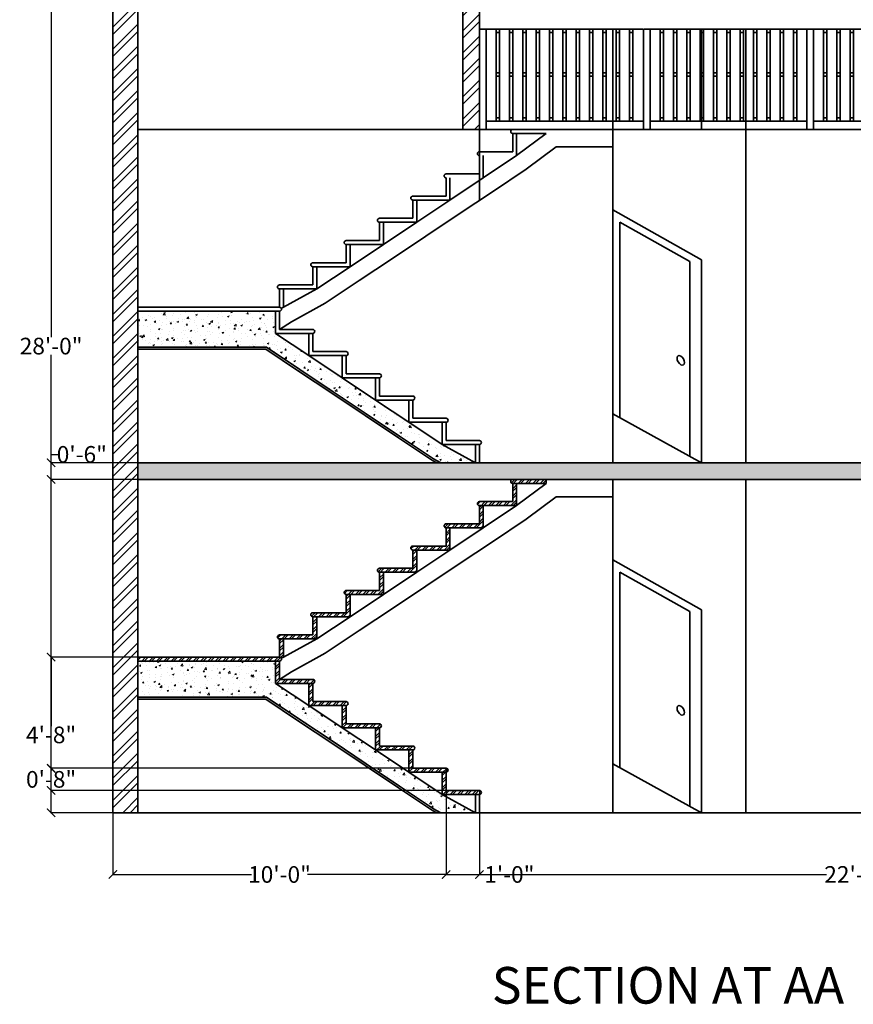
# Model space of a CAD drawing. Units: inches. Extents: x 2278 to 7495, y -71 to 1198.
# Tile 39 of 44: x 6954 to 7254, y 85 to 439. Entities that reach past the tile are written whole.
import ezdxf

# ---------------------------------------------------------------- set-up
doc = ezdxf.new("R2010")
doc.units = ezdxf.units.IN
doc.header["$MEASUREMENT"] = 0
for name, color, linetype, lineweight in [('A-ANNO-DIMS', 2, 'Continuous', 18), ('A-ANNO-TEXT', 7, 'Continuous', 25), ('A-SECT', 7, 'Continuous', 35), ('A-SECT-PATT', 8, 'Continuous', 13)]:
    doc.layers.add(name, color=color, linetype=linetype, lineweight=lineweight)
doc.styles.add('ATTR', font='romans.shx', dxfattribs={"width": 0.8, "height": 0.7})
doc.styles.get("Standard").update_dxf_attribs({"font": 'arial.ttf'})
doc.dimstyles.get("Standard").update_dxf_attribs({"dimtxt": 6, "dimasz": 3, "dimexe": 0.18, "dimexo": 0.0625, "dimgap": 0.09, "dimtad": 0, "dimtih": 1, "dimtoh": 1, "dimdec": 0, "dimzin": 0, "dimdsep": 46, "dimlunit": 3, "dimtxsty": 'Standard', "dimblk": 'ARCHTICK', "dimcen": 0.09, "dimadec": 0, "dimazin": 0, "dimtfac": 1, "dimtdec": 0, "dimtofl": 0, "dimtmove": 0, "dimatfit": 3, "dimfxl": 1, "dimtolj": 1, "dimtzin": 0, "dimarcsym": 0})
pattern_1 = [(45, (0, 155.5801), (-1.3258252, 1.3258252), []), (45, (0.8839, 155.5801), (-1.3258252, 1.3258252), [])]
pattern_2 = [(50, (0, 155.58), (5.7380815, -0.502017), [0.6, -6.6]), (355, (0, 155.58), (-1.1100107, 6.017537), [0.48, -5.28]), (100.45144, (0.478, 155.538), (4.6280708, 5.51552), [0.5099215, -5.609137]), (46.1842, (0, 157.18), (8.5379306, -1.324154), [0.9, -9.9]), (96.63564, (0.7115, 157.07), (7.477296, 7.792949), [0.764883, -8.41371]), (351.18416, (0, 157.18), (7.477296, 7.792949), [0.72, -7.92]), (21, (0.8, 156.78), (4.7752564, -3.220951), [0.6, -6.6]), (326, (0.8, 156.78), (1.9465227, 5.8012004), [0.48, -5.28]), (71.451445, (1.198, 156.5117), (6.721779, 2.5802492), [0.5099215, -5.609137]), (37.5, (0, 155.5801), (0.09727884, 2.66315083), [0, -5.216, 0, -5.36, 0, -5.3]), (7.5, (0, 155.58), (2.1045563, 3.1552937), [0, -3.056, 0, -5.096, 0, -2.02]), (327.5, (-1.784, 155.5801), (4.2705795, -0.180439), [0, -2, 0, -6.24, 0, -8.28]), (317.5, (-2.584, 155.58), (4.6654894, 0.8008399), [0, -2.6, 0, -4.144, 0, -5.88])]

# ---------------------------------------------------------------- blocks, each defined once
blk = doc.blocks.new('Fence 2 EV')
for p, q in [((0, 60), (0, 0)), ((0.001, 60.008), (98.001, 60.008)), ((4, 0.002), (4, 60)), ((10, 60), (10, 5.002)), ((12, 60), (12, 5.002)), ((18, 5.002), (18, 60)), ((20, 60), (20, 5.002)), ((25.999, 5.002), (25.999, 60)), ((27.999, 60), (27.999, 5.002)), ((33.999, 5.002), (33.999, 60)), ((35.999, 60), (35.999, 5.002)), ((41.999, 5.002), (41.999, 60)), ((43.999, 60), (43.999, 5.002)), ((49.999, 5.002), (49.999, 60)), ((51.998, 60), (51.998, 5.002)), ((57.998, 5.002), (57.998, 60)), ((59.998, 60), (59.998, 5.002)), ((65.998, 5.002), (65.998, 60)), ((67.998, 60), (67.998, 5.002)), ((73.998, 5.002), (73.998, 60)), ((75.997, 60), (75.997, 5.002)), ((81.997, 5.002), (81.997, 60)), ((83.997, 60), (83.997, 5.002)), ((89.997, 5.002), (89.997, 60)), ((91.997, 60), (91.997, 5.002)), ((10, 58), (12, 58)), ((18, 58), (20, 58)), ((25.999, 58), (27.999, 58)), ((33.999, 58), (35.999, 58)), ((41.999, 58), (43.999, 58)), ((49.999, 58), (51.998, 58)), ((57.998, 58), (59.998, 58)), ((65.998, 58), (67.998, 58)), ((73.998, 58), (75.997, 58)), ((81.997, 58), (83.997, 58)), ((89.997, 58), (91.997, 58)), ((10, 34.001), (12, 34.001)), ((10, 32.001), (12, 32.001)), ((18, 34.001), (20, 34.001)), ((18, 32.001), (20, 32.001)), ((25.999, 34.001), (27.999, 34.001)), ((25.999, 32.001), (27.999, 32.001)), ((33.999, 34.001), (35.999, 34.001)), ((33.999, 32.001), (35.999, 32.001)), ((41.999, 34.001), (43.999, 34.001)), ((41.999, 32.001), (43.999, 32.001)), ((49.999, 34.001), (51.998, 34.001)), ((49.999, 32.001), (51.998, 32.001)), ((57.998, 34.001), (59.998, 34.001)), ((57.998, 32.001), (59.998, 32.001)), ((65.998, 34.001), (67.998, 34.001)), ((65.998, 32.001), (67.998, 32.001)), ((73.998, 34.001), (75.997, 34.001)), ((73.998, 32.001), (75.997, 32.001)), ((81.997, 34.001), (83.997, 34.001)), ((81.997, 32.001), (83.997, 32.001)), ((89.997, 34.001), (91.997, 34.001)), ((89.997, 32.001), (91.997, 32.001)), ((10, 7.002), (12, 7.002)), ((18, 7.002), (20, 7.002)), ((25.999, 7.002), (27.999, 7.002)), ((33.999, 7.002), (35.999, 7.002)), ((41.999, 7.002), (43.999, 7.002)), ((49.999, 7.002), (51.998, 7.002)), ((57.998, 7.002), (59.998, 7.002)), ((65.998, 7.002), (67.998, 7.002)), ((73.998, 7.002), (75.997, 7.002)), ((81.997, 7.002), (83.997, 7.002)), ((89.997, 7.002), (91.997, 7.002)), ((0, 0.002), (4, 0.002)), ((97.997, 5.002), (4, 5.002))]:
    blk.add_line(p, q)
at = {"style": 'ATTR', "width": 0.8, "flags": 9}
blk.add_attdef('ESTCODE', (0, 0), '', height=0.0196, dxfattribs=at)
blk = doc.blocks.new('_ArchTick')
at = {"color": 0, "linetype": 'ByBlock', "const_width": 0.15}
blk.add_lwpolyline([(-0.5, -0.5), (0.5, 0.5)], dxfattribs=at)
blk = doc.blocks.new('*D113')
at = {"layer": 'A-ANNO-DIMS', "color": 0, "lineweight": -2, "transparency": 16777216}
for p, q in [((7119.18, 489.83), (7412.55, 489.83)), ((7412.37, 489.83), (7412.37, 447.99)), ((7412.37, 399.83), (7412.37, 441.68)), ((7119.18, 399.83), (7412.55, 399.83))]:
    blk.add_line(p, q, dxfattribs=at)
at = {"layer": 'Defpoints', "color": 0, "transparency": 16777216}
for p in [(7119.12, 489.83), (7412.37, 489.83), (7119.12, 399.83)]:
    blk.add_point(p, dxfattribs=at)
at = {"layer": 'A-ANNO-DIMS', "color": 0, "lineweight": -2, "transparency": 16777216, "xscale": 3, "yscale": 3, "zscale": 3}
for p, rotation in [((7412.37, 489.83), 90), ((7412.37, 399.83), 270)]:
    blk.add_blockref('_ArchTick', p, dxfattribs=dict(at, rotation=rotation))
at = {"layer": 'A-ANNO-DIMS', "color": 0, "transparency": 16777216, "insert": (7412.37, 444.83), "char_height": 6, "attachment_point": 5}
blk.add_mtext('\\A1;7\'-6"', dxfattribs=at)
blk = doc.blocks.new('*D114')
at = {"layer": 'A-ANNO-DIMS', "color": 0, "lineweight": -2, "transparency": 16777216}
for p, q in [((6987.05, 489.83), (6964.69, 489.83)), ((6964.87, 489.83), (6964.87, 324.99)), ((6964.87, 153.83), (6964.87, 318.68)), ((6987.05, 153.83), (6964.69, 153.83))]:
    blk.add_line(p, q, dxfattribs=at)
at = {"layer": 'Defpoints', "color": 0, "transparency": 16777216}
for p in [(6964.87, 489.83), (6987.12, 489.83), (6987.12, 153.83)]:
    blk.add_point(p, dxfattribs=at)
at = {"layer": 'A-ANNO-DIMS', "color": 0, "lineweight": -2, "transparency": 16777216, "xscale": 3, "yscale": 3, "zscale": 3}
for p, rotation in [((6964.87, 489.83), 90), ((6964.87, 153.83), 270)]:
    blk.add_blockref('_ArchTick', p, dxfattribs=dict(at, rotation=rotation))
at = {"layer": 'A-ANNO-DIMS', "color": 0, "transparency": 16777216, "insert": (6964.87, 321.83), "char_height": 6, "attachment_point": 5}
blk.add_mtext('\\A1;28\'-0"', dxfattribs=at)
blk = doc.blocks.new('*D115')
at = {"layer": 'A-ANNO-DIMS', "color": 0, "lineweight": -2, "transparency": 16777216}
for p, q in [((6996.05, 209.83), (6964.69, 209.83)), ((6964.87, 209.83), (6964.87, 184.99)), ((6964.87, 153.83), (6964.87, 178.68)), ((6996.05, 153.83), (6964.69, 153.83))]:
    blk.add_line(p, q, dxfattribs=at)
at = {"layer": 'Defpoints', "color": 0, "transparency": 16777216}
for p in [(6964.87, 209.83), (6996.12, 209.83), (6996.12, 153.83)]:
    blk.add_point(p, dxfattribs=at)
at = {"layer": 'A-ANNO-DIMS', "color": 0, "lineweight": -2, "transparency": 16777216, "xscale": 3, "yscale": 3, "zscale": 3}
for p, rotation in [((6964.87, 209.83), 90), ((6964.87, 153.83), 270)]:
    blk.add_blockref('_ArchTick', p, dxfattribs=dict(at, rotation=rotation))
at = {"layer": 'A-ANNO-DIMS', "color": 0, "transparency": 16777216, "insert": (6964.87, 181.83), "char_height": 6, "attachment_point": 5}
blk.add_mtext('\\A1;4\'-8"', dxfattribs=at)
blk = doc.blocks.new('*D116')
at = {"layer": 'A-ANNO-DIMS', "color": 0, "lineweight": -2, "transparency": 16777216}
for p, q in [((6964.87, 279.83), (6964.87, 282.83)), ((6964.87, 282.83), (6967.87, 282.83)), ((6996.05, 279.83), (6964.69, 279.83)), ((6964.87, 273.83), (6964.87, 279.83)), ((6996.05, 273.83), (6964.69, 273.83))]:
    blk.add_line(p, q, dxfattribs=at)
at = {"layer": 'Defpoints', "color": 0, "transparency": 16777216}
for p in [(6964.87, 279.83), (6996.12, 279.83), (6996.12, 273.83)]:
    blk.add_point(p, dxfattribs=at)
at = {"layer": 'A-ANNO-DIMS', "color": 0, "lineweight": -2, "transparency": 16777216, "xscale": 3, "yscale": 3, "zscale": 3}
for p, rotation in [((6964.87, 279.83), 90), ((6964.87, 273.83), 270)]:
    blk.add_blockref('_ArchTick', p, dxfattribs=dict(at, rotation=rotation))
at = {"layer": 'A-ANNO-DIMS', "color": 0, "transparency": 16777216, "insert": (6975.93, 282.83), "char_height": 6, "attachment_point": 5}
blk.add_mtext('\\A1;0\'-6"', dxfattribs=at)
blk = doc.blocks.new('*D117')
at = {"layer": 'A-ANNO-DIMS', "color": 0, "lineweight": -2, "transparency": 16777216}
for p, q in [((7107.05, 169.83), (6964.69, 169.83)), ((6964.87, 169.83), (6964.87, 168.99)), ((7119.05, 161.83), (6964.69, 161.83)), ((6964.87, 161.83), (6964.87, 162.68))]:
    blk.add_line(p, q, dxfattribs=at)
at = {"layer": 'Defpoints', "color": 0, "transparency": 16777216}
for p in [(6964.87, 169.83), (7107.12, 169.83), (7119.12, 161.83)]:
    blk.add_point(p, dxfattribs=at)
at = {"layer": 'A-ANNO-DIMS', "color": 0, "lineweight": -2, "transparency": 16777216, "xscale": 3, "yscale": 3, "zscale": 3}
for p, rotation in [((6964.87, 169.83), 90), ((6964.87, 161.83), 270)]:
    blk.add_blockref('_ArchTick', p, dxfattribs=dict(at, rotation=rotation))
at = {"layer": 'A-ANNO-DIMS', "color": 0, "transparency": 16777216, "insert": (6964.87, 165.83), "char_height": 6, "attachment_point": 5}
blk.add_mtext('\\A1;0\'-8"', dxfattribs=at)
blk = doc.blocks.new('*D118')
at = {"layer": 'A-ANNO-DIMS', "color": 0, "lineweight": -2, "transparency": 16777216}
for p, q in [((7107.12, 169.77), (7107.12, 131.4)), ((6987.12, 153.77), (6987.12, 131.4)), ((6987.12, 131.58), (7037, 131.58)), ((7107.12, 131.58), (7057.23, 131.58))]:
    blk.add_line(p, q, dxfattribs=at)
at = {"layer": 'Defpoints', "color": 0, "transparency": 16777216}
for p in [(7107.12, 169.83), (6987.12, 153.83), (7107.12, 131.58)]:
    blk.add_point(p, dxfattribs=at)
at = {"layer": 'A-ANNO-DIMS', "color": 0, "lineweight": -2, "transparency": 16777216, "xscale": 3, "yscale": 3, "zscale": 3, "rotation": 180}
blk.add_blockref('_ArchTick', (6987.12, 131.58), dxfattribs=at)
at = {"layer": 'A-ANNO-DIMS', "color": 0, "lineweight": -2, "transparency": 16777216, "xscale": 3, "yscale": 3, "zscale": 3}
blk.add_blockref('_ArchTick', (7107.12, 131.58), dxfattribs=at)
at = {"layer": 'A-ANNO-DIMS', "color": 0, "transparency": 16777216, "insert": (7047.12, 131.58), "char_height": 6, "attachment_point": 5}
blk.add_mtext('\\A1;10\'-0"', dxfattribs=at)
blk = doc.blocks.new('*D119')
at = {"layer": 'A-ANNO-DIMS', "color": 0, "lineweight": -2, "transparency": 16777216}
for p, q in [((7107.12, 169.77), (7107.12, 131.4)), ((7119.12, 161.77), (7119.12, 131.4)), ((7107.12, 131.58), (7119.12, 131.58)), ((7119.12, 131.58), (7122.12, 131.58))]:
    blk.add_line(p, q, dxfattribs=at)
at = {"layer": 'Defpoints', "color": 0, "transparency": 16777216}
for p in [(7107.12, 169.83), (7119.12, 161.83), (7119.12, 131.58)]:
    blk.add_point(p, dxfattribs=at)
at = {"layer": 'A-ANNO-DIMS', "color": 0, "lineweight": -2, "transparency": 16777216, "xscale": 3, "yscale": 3, "zscale": 3, "rotation": 180}
blk.add_blockref('_ArchTick', (7107.12, 131.58), dxfattribs=at)
at = {"layer": 'A-ANNO-DIMS', "color": 0, "lineweight": -2, "transparency": 16777216, "xscale": 3, "yscale": 3, "zscale": 3}
blk.add_blockref('_ArchTick', (7119.12, 131.58), dxfattribs=at)
at = {"layer": 'A-ANNO-DIMS', "color": 0, "transparency": 16777216, "insert": (7129.9, 131.58), "char_height": 6, "attachment_point": 5}
blk.add_mtext('\\A1;1\'-0"', dxfattribs=at)
blk = doc.blocks.new('*D120')
at = {"layer": 'A-ANNO-DIMS', "color": 0, "lineweight": -2, "transparency": 16777216}
for p, q in [((7119.12, 161.77), (7119.12, 131.4)), ((7390.12, 153.77), (7390.12, 131.4)), ((7119.12, 131.58), (7244.17, 131.58)), ((7390.12, 131.58), (7265.06, 131.58))]:
    blk.add_line(p, q, dxfattribs=at)
at = {"layer": 'Defpoints', "color": 0, "transparency": 16777216}
for p in [(7119.12, 161.83), (7390.12, 153.83), (7390.12, 131.58)]:
    blk.add_point(p, dxfattribs=at)
at = {"layer": 'A-ANNO-DIMS', "color": 0, "lineweight": -2, "transparency": 16777216, "xscale": 3, "yscale": 3, "zscale": 3, "rotation": 180}
blk.add_blockref('_ArchTick', (7119.12, 131.58), dxfattribs=at)
at = {"layer": 'A-ANNO-DIMS', "color": 0, "lineweight": -2, "transparency": 16777216, "xscale": 3, "yscale": 3, "zscale": 3}
blk.add_blockref('_ArchTick', (7390.12, 131.58), dxfattribs=at)
at = {"layer": 'A-ANNO-DIMS', "color": 0, "transparency": 16777216, "insert": (7254.62, 131.58), "char_height": 6, "attachment_point": 5}
blk.add_mtext('\\A1;22\'-7"', dxfattribs=at)
blk = doc.blocks.new('*D122')
at = {"layer": 'A-ANNO-DIMS', "color": 0, "lineweight": -2, "transparency": 16777216}
for p, q in [((7119.12, 489.9), (7119.12, 512.26)), ((7119.12, 512.08), (7244.17, 512.08)), ((7390.11, 512.08), (7265.06, 512.08)), ((7390.11, 435.95), (7390.11, 512.26))]:
    blk.add_line(p, q, dxfattribs=at)
at = {"layer": 'Defpoints', "color": 0, "transparency": 16777216}
for p in [(7390.11, 512.08), (7119.12, 489.83), (7390.11, 435.89)]:
    blk.add_point(p, dxfattribs=at)
at = {"layer": 'A-ANNO-DIMS', "color": 0, "lineweight": -2, "transparency": 16777216, "xscale": 3, "yscale": 3, "zscale": 3, "rotation": 180}
blk.add_blockref('_ArchTick', (7119.12, 512.08), dxfattribs=at)
at = {"layer": 'A-ANNO-DIMS', "color": 0, "lineweight": -2, "transparency": 16777216, "xscale": 3, "yscale": 3, "zscale": 3}
blk.add_blockref('_ArchTick', (7390.11, 512.08), dxfattribs=at)
at = {"layer": 'A-ANNO-DIMS', "color": 0, "transparency": 16777216, "insert": (7254.61, 512.08), "char_height": 6, "attachment_point": 5}
blk.add_mtext('\\A1;22\'-7"', dxfattribs=at)

msp = doc.modelspace()

# ---------------------------------------------------------------- hatches: boundary and pattern name
at = {"layer": 'A-SECT-PATT', "transparency": 33554687}
h = msp.add_hatch(dxfattribs=at)
h.set_pattern_fill('ANSI32', color=256, scale=15)
h.set_pattern_definition([(45, (0, 155.58), (-3.9774756, 3.9774756), []), (45, (2.6517, 155.58), (-3.9774756, 3.9774756), [])])
h.paths.add_polyline_path([(6996.12, 489.83), (6987.12, 489.83), (6987.12, 153.83), (6996.12, 153.83)])
h.paths.add_polyline_path([(7390.12, 399.83), (7381.12, 399.83), (7381.12, 153.83), (7390.12, 153.83)])
h.paths.add_polyline_path([(7119.12, 483.83), (7119.12, 489.83), (7113.12, 489.83), (7113.12, 399.83), (7119.12, 399.83)])
h = msp.add_hatch(dxfattribs=at)
h.set_pattern_fill('AR-CONC', color=256, scale=0.8)
h.set_pattern_definition(pattern_2)
h.paths.add_polyline_path([(7045.72, 334.4), (6996.12, 334.4), (6996.12, 321.4), (7042.39, 321.4), (7054.39, 313.4), (7066.39, 305.4), (7078.39, 297.4), (7090.39, 289.4), (7102.61, 281.26), (7105.21, 279.83), (7117.72, 279.83), (7105.72, 286.4), (7093.72, 294.4), (7081.72, 302.4), (7069.72, 310.4), (7057.72, 318.4), (7045.72, 326.4)])
h = msp.add_hatch(dxfattribs=at)
h.set_pattern_fill('AR-CONC', color=256, scale=0.8)
h.set_pattern_definition([(50, (0, 0), (5.7380815, -0.502017), [0.6, -6.6]), (355, (0, 0), (-1.1100107, 6.017537), [0.48, -5.28]), (100.451444, (0.478, -0.042), (4.6280708, 5.51552), [0.5099215, -5.609137]), (46.1842, (0, 1.6), (8.5379306, -1.324154), [0.9, -9.9]), (96.63564, (0.7115, 1.49), (7.477296, 7.792949), [0.764883, -8.41371]), (351.18416, (0, 1.6), (7.477296, 7.792949), [0.72, -7.92]), (21, (0.8, 1.2), (4.7752564, -3.220951), [0.6, -6.6]), (326, (0.8, 1.2), (1.9465227, 5.8012004), [0.48, -5.28]), (71.451445, (1.198, 0.9316), (6.721779, 2.5802492), [0.5099215, -5.609137]), (37.5, (0, 0), (0.09727884, 2.66315083), [0, -5.216, 0, -5.36, 0, -5.3]), (7.5, (0, 0), (2.1045563, 3.1552937), [0, -3.056, 0, -5.096, 0, -2.02]), (327.5, (-1.784, 0), (4.2705795, -0.180439), [0, -2, 0, -6.24, 0, -8.28]), (317.5, (-2.584, 0), (4.6654894, 0.8008399), [0, -2.6, 0, -4.144, 0, -5.88])])
h.paths.add_polyline_path([(7381.12, 279.83), (6996.12, 279.83), (6996.12, 273.83), (7131.12, 273.83), (7143.12, 273.83), (7167.12, 273.83), (7381.12, 273.83)])
h = msp.add_hatch(dxfattribs=at)
h.set_pattern_fill('ANSI32', color=256, scale=5)
h.set_pattern_definition(pattern_1)
h.paths.add_polyline_path([(7143.12, 273.83), (7131.12, 273.83, 1), (7131.12, 272.4), (7143.12, 272.4)])
h = msp.add_hatch(dxfattribs=at)
h.set_pattern_fill('ANSI32', color=256, scale=5)
h.set_pattern_definition(pattern_1)
h.paths.add_polyline_path([(7107.12, 169.83), (7095.12, 169.83), (7095.12, 176.4), (7093.72, 176.4), (7093.72, 168.4), (7107.12, 168.4, 1)])
h.paths.add_polyline_path([(7107.12, 168.4), (7105.72, 168.4), (7105.72, 160.4), (7119.12, 160.4, 1), (7119.12, 161.83), (7107.12, 161.83)])
h.paths.add_polyline_path([(7095.12, 177.83), (7083.12, 177.83), (7083.12, 184.4), (7081.72, 184.4), (7081.72, 176.4), (7095.12, 176.4, 1)])
h.paths.add_polyline_path([(7083.12, 185.83), (7071.12, 185.83), (7071.12, 192.4), (7069.72, 192.4), (7069.72, 184.4), (7083.12, 184.4, 1)])
h.paths.add_polyline_path([(7071.12, 193.83), (7059.12, 193.83), (7059.12, 200.4), (7057.72, 200.4), (7057.72, 192.4), (7071.12, 192.4, 1)])
h.paths.add_polyline_path([(7059.12, 201.83), (7047.12, 201.83), (7047.12, 208.4), (7045.72, 208.4), (7045.72, 200.4), (7059.12, 200.4, 1)])
h.paths.add_polyline_path([(7047.12, 209.83), (7035.12, 209.83), (6996.12, 209.83), (6996.12, 208.4), (7047.12, 208.4, 1)])
h.paths.add_polyline_path([(7048.52, 216.4), (7047.12, 216.4), (7047.12, 209.83, -0.289905), (7047.76, 209.42), (7048.52, 209.83)])
h.paths.add_polyline_path([(7060.52, 224.4), (7059.12, 224.4), (7059.12, 217.83), (7047.12, 217.83, 1), (7047.12, 216.4), (7048.52, 216.4), (7060.52, 216.4)])
h.paths.add_polyline_path([(7072.52, 232.4), (7071.12, 232.4), (7071.12, 225.83), (7059.12, 225.83, 1), (7059.12, 224.4), (7060.52, 224.4), (7072.52, 224.4)])
h.paths.add_polyline_path([(7084.52, 240.4), (7083.12, 240.4), (7083.12, 233.83), (7071.12, 233.83, 1), (7071.12, 232.4), (7072.52, 232.4), (7084.52, 232.4)])
h.paths.add_polyline_path([(7096.52, 248.4), (7095.12, 248.4), (7095.12, 241.83), (7083.12, 241.83, 1), (7083.12, 240.4), (7084.52, 240.4), (7096.52, 240.4)])
h.paths.add_polyline_path([(7108.52, 256.4), (7107.12, 256.4), (7107.12, 249.83), (7095.12, 249.83, 1), (7095.12, 248.4), (7096.52, 248.4), (7108.52, 248.4)])
h.paths.add_polyline_path([(7120.52, 264.4), (7119.12, 264.4), (7119.12, 257.83), (7107.12, 257.83, 1), (7107.12, 256.4), (7120.52, 256.4)])
h.paths.add_polyline_path([(7132.52, 272.4), (7131.12, 272.4), (7131.12, 265.83), (7119.12, 265.83, 1), (7119.12, 264.4), (7120.52, 264.4), (7132.52, 264.4)])
h = msp.add_hatch(dxfattribs=at)
h.set_pattern_fill('AR-CONC', color=256, scale=0.8)
h.set_pattern_definition(pattern_2)
h.paths.add_polyline_path([(7045.72, 208.4), (6996.12, 208.4), (6996.12, 195.4), (7042.39, 195.4), (7054.39, 187.4), (7066.39, 179.4), (7078.39, 171.4), (7090.39, 163.4), (7102.61, 155.26), (7105.21, 153.83), (7117.72, 153.83), (7105.72, 160.4), (7093.72, 168.4), (7081.72, 176.4), (7069.72, 184.4), (7057.72, 192.4), (7045.72, 200.4)])

# ---------------------------------------------------------------- linework, layer by layer
at = {"layer": 'A-SECT'}
for p, q in [((6987.12, 153.83), (6987.12, 489.83)), ((6996.12, 153.83), (6996.12, 489.83)), ((7113.12, 399.83), (7113.12, 489.83)), ((7119.12, 489.83), (7119.12, 374.25)), ((7119.12, 399.83), (7119.12, 483.83)), ((7167.12, 435.89), (7167.12, 279.83)), ((7199.04, 399.83), (7199.04, 435.89)), ((7215.12, 435.89), (7215.12, 279.83)), ((6996.12, 399.83), (7390.12, 399.83)), ((7131.12, 399.83), (7143.12, 399.83)), ((7131.12, 398.4), (7131.12, 391.83)), ((7143.12, 398.4), (7131.12, 398.4)), ((7132.52, 398.4), (7132.52, 390.4)), ((7167.12, 393.61), (7167.12, 399.83)), ((7146.73, 393.61), (7167.12, 393.61)), ((7119.12, 391.83), (7131.12, 391.83)), ((7119.12, 390.4), (7119.12, 383.83)), ((7120.52, 390.4), (7120.52, 382.4)), ((7107.12, 383.83), (7119.12, 383.83)), ((7107.12, 382.4), (7107.12, 375.83)), ((7108.52, 382.4), (7108.52, 374.4)), ((7095.12, 375.83), (7107.12, 375.83)), ((7095.12, 374.4), (7095.12, 367.83)), ((7108.52, 374.4), (7095.12, 374.4)), ((7096.52, 374.4), (7096.52, 366.4)), ((7167.12, 297.43), (7167.12, 370.92)), ((7167.12, 370.92), (7199.04, 352.92)), ((7083.12, 367.83), (7095.12, 367.83)), ((7083.12, 366.4), (7083.12, 359.83)), ((7096.52, 366.4), (7083.12, 366.4)), ((7084.52, 366.4), (7084.52, 358.4)), ((7169.71, 366.46), (7194.85, 352.28)), ((7169.71, 295.93), (7169.71, 366.46)), ((7071.12, 359.83), (7083.12, 359.83)), ((7071.12, 358.4), (7071.12, 351.83)), ((7084.52, 358.4), (7071.12, 358.4)), ((7072.52, 358.4), (7072.52, 350.4)), ((7059.12, 351.83), (7071.12, 351.83)), ((7194.85, 282.14), (7194.85, 352.28)), ((7199.04, 279.83), (7199.04, 352.92)), ((7059.12, 350.4), (7059.12, 343.83)), ((7072.52, 350.4), (7059.12, 350.4)), ((7060.52, 350.4), (7060.52, 342.4)), ((7047.12, 343.83), (7059.12, 343.83)), ((7047.12, 342.4), (7047.12, 335.83)), ((7060.52, 342.4), (7047.12, 342.4)), ((7048.52, 342.4), (7048.52, 335.83)), ((7035.12, 335.83), (6996.12, 335.83)), ((7047.12, 334.4), (6996.12, 334.4)), ((7047.12, 335.83), (7035.12, 335.83)), ((7045.72, 334.4), (7045.72, 326.4)), ((7047.12, 334.4), (7047.12, 327.83)), ((7048.52, 335.83), (7047.76, 335.42)), ((7051.39, 330.57), (7047.12, 327.83)), ((7059.12, 326.4), (7045.72, 326.4)), ((7059.12, 327.83), (7047.12, 327.83)), ((7057.72, 326.4), (7057.72, 318.4)), ((7059.12, 326.4), (7059.12, 319.83)), ((7042.39, 321.4), (6996.12, 321.4)), ((7042.18, 320.7), (6996.12, 320.7)), ((7071.12, 319.83), (7059.12, 319.83)), ((7071.12, 318.4), (7057.72, 318.4)), ((7069.72, 318.4), (7069.72, 310.4)), ((7071.12, 318.4), (7071.12, 311.83)), ((7083.12, 310.4), (7069.72, 310.4)), ((7083.12, 311.83), (7071.12, 311.83)), ((7081.72, 310.4), (7081.72, 302.4)), ((7083.12, 310.4), (7083.12, 303.83)), ((7095.12, 302.4), (7081.72, 302.4)), ((7081.72, 302.4), (7081.72, 302.4)), ((7095.12, 303.83), (7083.12, 303.83)), ((7093.72, 302.4), (7093.72, 294.4)), ((7095.12, 302.4), (7095.12, 295.83)), ((7107.12, 294.4), (7093.72, 294.4)), ((7107.12, 295.83), (7095.12, 295.83)), ((7105.72, 294.4), (7105.72, 286.4)), ((7107.12, 294.4), (7107.12, 287.83)), ((7199.04, 279.83), (7167.12, 297.43)), ((7119.12, 287.83), (7107.12, 287.83)), ((7119.12, 286.4), (7105.72, 286.4)), ((7117.72, 286.4), (7117.72, 279.83)), ((7119.12, 286.4), (7119.12, 279.83)), ((6996.12, 279.83), (7381.12, 279.83)), ((7131.12, 273.83), (6996.12, 273.83)), ((7131.12, 273.83), (7143.12, 273.83)), ((7143.12, 273.83), (7167.12, 273.83)), ((7143.12, 272.4), (7143.12, 273.83)), ((7167.12, 273.83), (7381.12, 273.83)), ((7167.12, 267.61), (7167.12, 273.83)), ((7167.12, 273.83), (7167.12, 153.83)), ((7215.12, 273.83), (7215.12, 153.83)), ((7131.12, 272.4), (7131.12, 265.83)), ((7143.12, 272.4), (7131.12, 272.4)), ((7132.52, 272.4), (7132.52, 264.4)), ((7146.73, 267.61), (7167.12, 267.61)), ((7119.12, 265.83), (7131.12, 265.83)), ((7119.12, 264.4), (7119.12, 257.83)), ((7132.52, 264.4), (7119.12, 264.4)), ((7120.52, 264.4), (7120.52, 256.4)), ((7107.12, 257.83), (7119.12, 257.83)), ((7107.12, 256.4), (7107.12, 249.83)), ((7120.52, 256.4), (7107.12, 256.4)), ((7108.52, 256.4), (7108.52, 248.4)), ((7095.12, 249.83), (7107.12, 249.83)), ((7095.12, 248.4), (7095.12, 241.83)), ((7108.52, 248.4), (7095.12, 248.4)), ((7096.52, 248.4), (7096.52, 240.4)), ((7167.12, 171.43), (7167.12, 244.92)), ((7167.12, 244.92), (7199.04, 226.92)), ((7083.12, 241.83), (7095.12, 241.83)), ((7083.12, 240.4), (7083.12, 233.83)), ((7096.52, 240.4), (7083.12, 240.4)), ((7084.52, 240.4), (7084.52, 232.4)), ((7169.71, 240.46), (7194.85, 226.28)), ((7169.71, 169.93), (7169.71, 240.46)), ((7071.12, 233.83), (7083.12, 233.83)), ((7071.12, 232.4), (7071.12, 225.83)), ((7084.52, 232.4), (7071.12, 232.4)), ((7072.52, 232.4), (7072.52, 224.4)), ((7199.04, 153.83), (7199.04, 226.92)), ((7059.12, 225.83), (7071.12, 225.83)), ((7059.12, 224.4), (7059.12, 217.83)), ((7072.52, 224.4), (7059.12, 224.4)), ((7060.52, 224.4), (7060.52, 216.4)), ((7194.85, 156.14), (7194.85, 226.28)), ((7047.12, 217.83), (7059.12, 217.83)), ((7047.12, 216.4), (7047.12, 209.83)), ((7060.52, 216.4), (7047.12, 216.4)), ((7048.52, 216.4), (7048.52, 209.83)), ((7035.12, 209.83), (6996.12, 209.83)), ((7047.12, 209.83), (7035.12, 209.83)), ((7048.52, 209.83), (7047.76, 209.42)), ((7047.12, 208.4), (6996.12, 208.4)), ((7045.72, 208.4), (7045.72, 200.4)), ((7047.12, 208.4), (7047.12, 201.83)), ((7051.39, 204.57), (7047.12, 201.83)), ((7059.12, 200.4), (7045.72, 200.4)), ((7059.12, 201.83), (7047.12, 201.83)), ((7057.72, 200.4), (7057.72, 192.4)), ((7059.12, 200.4), (7059.12, 193.83)), ((7042.39, 195.4), (6996.12, 195.4)), ((7042.18, 194.7), (6996.12, 194.7)), ((7071.12, 192.4), (7057.72, 192.4)), ((7071.12, 193.83), (7059.12, 193.83)), ((7069.72, 192.4), (7069.72, 184.4)), ((7071.12, 192.4), (7071.12, 185.83)), ((7083.12, 184.4), (7069.72, 184.4)), ((7083.12, 185.83), (7071.12, 185.83)), ((7081.72, 184.4), (7081.72, 176.4)), ((7083.12, 184.4), (7083.12, 177.83)), ((7095.12, 177.83), (7083.12, 177.83)), ((7095.12, 176.4), (7081.72, 176.4)), ((7081.72, 176.4), (7081.72, 176.4)), ((7093.72, 176.4), (7093.72, 168.4)), ((7095.12, 176.4), (7095.12, 169.83)), ((7199.04, 153.83), (7167.12, 171.43)), ((7107.12, 168.4), (7093.72, 168.4)), ((7107.12, 169.83), (7095.12, 169.83)), ((7105.72, 168.4), (7105.72, 160.4)), ((7107.12, 168.4), (7107.12, 161.83)), ((7119.12, 160.4), (7105.72, 160.4)), ((7119.12, 161.83), (7107.12, 161.83)), ((7117.72, 160.4), (7117.72, 153.83)), ((7119.12, 160.4), (7119.12, 153.83)), ((6987.12, 153.83), (7390.12, 153.83))]:
    msp.add_line(p, q, dxfattribs=at)
for points in [[(7048.52, 335.83), (7060.52, 342.4), (7072.52, 350.4), (7084.52, 358.4), (7096.52, 366.4), (7108.52, 374.4), (7120.52, 382.4), (7132.52, 390.4), (7143.12, 398.4)], [(7051.39, 330.57), (7063.62, 337.26), (7075.84, 345.4), (7087.84, 353.4), (7099.84, 361.4), (7111.84, 369.4), (7123.84, 377.4), (7135.99, 385.5), (7146.73, 393.61)], [(7045.72, 326.4), (7057.72, 318.4), (7069.72, 310.4), (7081.72, 302.4), (7093.72, 294.4), (7105.72, 286.4), (7117.72, 279.83)], [(7042.18, 320.7), (7054, 312.82), (7066, 304.82), (7078, 296.82), (7090, 288.82), (7102.24, 280.66), (7103.75, 279.83)], [(7042.39, 321.4), (7054.39, 313.4), (7066.39, 305.4), (7078.39, 297.4), (7090.39, 289.4), (7102.61, 281.26), (7105.21, 279.83)], [(7048.52, 209.83), (7060.52, 216.4), (7072.52, 224.4), (7084.52, 232.4), (7096.52, 240.4), (7108.52, 248.4), (7120.52, 256.4), (7132.52, 264.4), (7143.12, 272.4)], [(7051.39, 204.57), (7063.62, 211.26), (7075.84, 219.4), (7087.84, 227.4), (7099.84, 235.4), (7111.84, 243.4), (7123.84, 251.4), (7135.99, 259.5), (7146.73, 267.61)], [(7045.72, 200.4), (7057.72, 192.4), (7069.72, 184.4), (7081.72, 176.4), (7093.72, 168.4), (7105.72, 160.4), (7117.72, 153.83)], [(7042.39, 195.4), (7054.39, 187.4), (7066.39, 179.4), (7078.39, 171.4), (7090.39, 163.4), (7102.61, 155.26), (7105.21, 153.83)], [(7042.18, 194.7), (7054, 186.82), (7066, 178.82), (7078, 170.82), (7090, 162.82), (7102.24, 154.66), (7103.75, 153.83)]]:
    msp.add_lwpolyline(points, dxfattribs=at)
for centre, start, end in [((7131.12, 399.11), 90, 270), ((7119.12, 391.11), 90, 270), ((7107.12, 383.11), 90, 270), ((7095.12, 375.11), 90, 270), ((7083.12, 367.11), 90, 270), ((7071.12, 359.11), 90, 270), ((7059.12, 351.11), 90, 270), ((7047.12, 343.11), 90, 270), ((7047.12, 335.11), 270, 90), ((7059.12, 327.11), 270, 90), ((7071.12, 319.11), 270, 90), ((7083.12, 311.11), 270, 90), ((7095.12, 303.11), 270, 90), ((7107.12, 295.11), 270, 90), ((7119.12, 287.11), 270, 90), ((7131.12, 273.11), 90, 270), ((7119.12, 265.11), 90, 270), ((7107.12, 257.11), 90, 270), ((7095.12, 249.11), 90, 270), ((7083.12, 241.11), 90, 270), ((7071.12, 233.11), 90, 270), ((7059.12, 225.11), 90, 270), ((7047.12, 217.11), 90, 270), ((7047.12, 209.11), 270, 90), ((7059.12, 201.11), 270, 90), ((7071.12, 193.11), 270, 90), ((7083.12, 185.11), 270, 90), ((7095.12, 177.11), 270, 90), ((7107.12, 169.11), 270, 90), ((7119.12, 161.11), 270, 90)]:
    msp.add_arc(centre, 0.718, start, end, dxfattribs=at)
for centre in [(7191.62, 316.66), (7191.62, 190.66)]:
    msp.add_ellipse(centre, major_axis=(0.95, -1.64), ratio=0.57735, dxfattribs=at)

# ---------------------------------------------------------------- block references
at = {"layer": 'A-SECT', "xscale": 0.600830084310023, "yscale": 0.600830084310023, "zscale": 0.600830084310023}
for p in [(7119.12, 399.83), (7178.18, 399.83), (7236.98, 399.83)]:
    msp.add_blockref('Fence 2 EV', p, dxfattribs=at)

# ---------------------------------------------------------------- texts
at = {"layer": 'A-ANNO-TEXT'}
msp.add_text('SECTION AT AA ', height=13.1927, dxfattribs=at).set_placement((7123.58, 85.07))

# ---------------------------------------------------------------- dimensions: what is measured, and where the dimension line sits
at = {"layer": 'A-ANNO-DIMS'}
for base, p1, p2, picture, middle in [((7390.11, 512.08), (7119.12, 489.83), (7390.11, 435.89), '*D122', (7254.61, 512.08)), ((7107.12, 131.58), (6987.12, 153.83), (7107.12, 169.83), '*D118', (7047.12, 131.58)), ((7119.12, 131.58), (7107.12, 169.83), (7119.12, 161.83), '*D119', (7129.9, 131.58)), ((7390.12, 131.58), (7119.12, 161.83), (7390.12, 153.83), '*D120', (7254.62, 131.58))]:
    dim = msp.add_linear_dim(base=base, p1=p1, p2=p2, dimstyle='Standard', override={"dimdec": 1, "dimlfac": 1, "dimrnd": 0, "dimzin": 1, "dimdsep": 46, "dimlunit": 4, "dimfrac": 2}, dxfattribs=at)
    dim.commit()
    dim.dimension.update_dxf_attribs({"geometry": picture, "text_midpoint": middle})
for base, p1, p2, picture, middle in [((6964.87, 489.83), (6987.12, 153.83), (6987.12, 489.83), '*D114', (6964.87, 321.83)), ((7412.37, 489.83), (7119.12, 399.83), (7119.12, 489.83), '*D113', (7412.37, 444.83)), ((6964.87, 279.83), (6996.12, 273.83), (6996.12, 279.83), '*D116', (6975.93, 282.83)), ((6964.87, 209.83), (6996.12, 153.83), (6996.12, 209.83), '*D115', (6964.87, 181.83)), ((6964.87, 169.83), (7119.12, 161.83), (7107.12, 169.83), '*D117', (6964.87, 165.83))]:
    dim = msp.add_linear_dim(base=base, p1=p1, p2=p2, angle=90, dimstyle='Standard', override={"dimdec": 1, "dimlfac": 1, "dimrnd": 0, "dimzin": 1, "dimdsep": 46, "dimlunit": 4, "dimfrac": 2}, dxfattribs=at)
    dim.commit()
    dim.dimension.update_dxf_attribs({"geometry": picture, "text_midpoint": middle})

doc.saveas('drawing.dxf')
